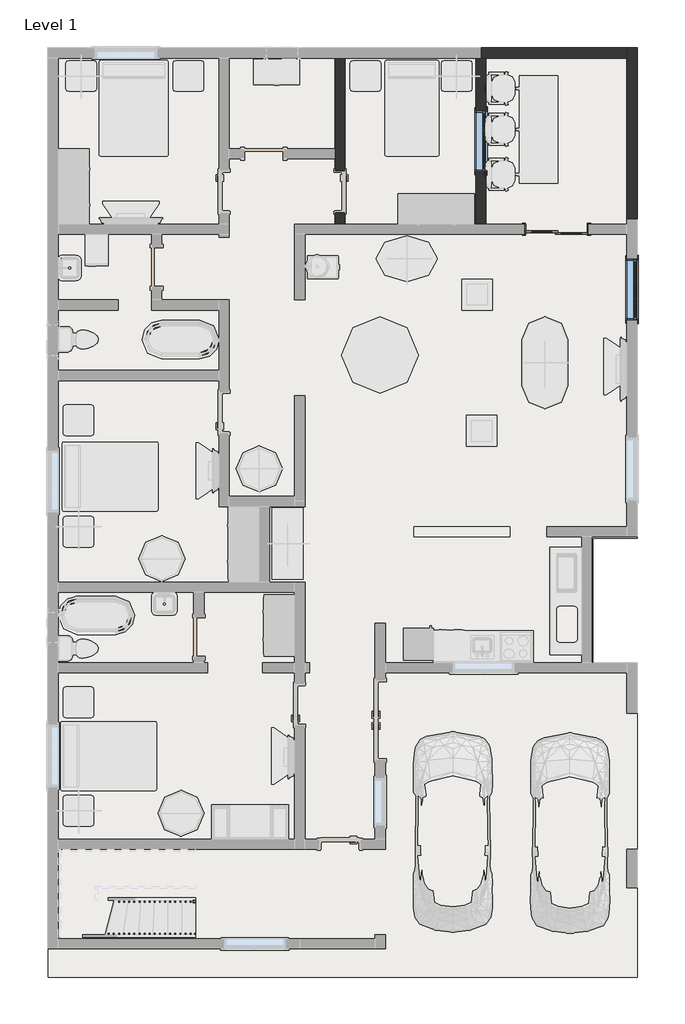
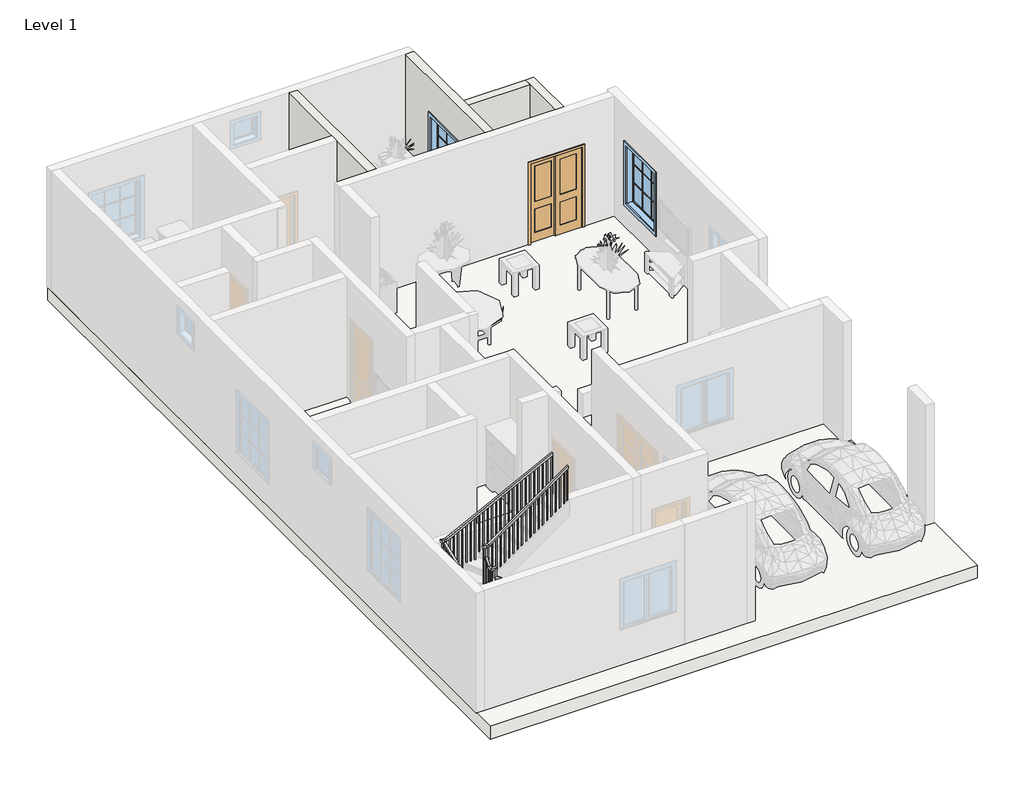
# One storey, part 2 of 3: 4 walls, 2 railings, 2 windows, 1 door, 1 slab.
"""IFC4 building model written with IfcOpenShell, lengths in millimetres."""

from ifc_helpers import new_model, si_unit, frame, origin, place, context, project, spatial, polyline, outline, extrude, faceted_brep, transform, mapped, element, save
from components import door_f9cb40a9, window_cfa1ffdd

model = new_model("IFC4")

# Units and contexts
model_context = context("Model", 3, world=origin())
ifc_project = project(units=[si_unit("LENGTHUNIT", "METRE", prefix="MILLI")], contexts=[model_context])

# Site, building, storey
site = spatial("IfcSite", under=ifc_project)
building = spatial("IfcBuilding", under=site)
storey = spatial("IfcBuildingStorey", under=building, Name="Level 1", Elevation=0.0)

# Door
placement = place(None, origin())
door_shape = door_f9cb40a9(model_context)
element("IfcDoor", 1, ObjectType="Door-Interior-Double-Sliding-2_Panel-Wood : 48\" x 80\"", at=placement, inside=storey, context=model_context, shape_type="MappedRepresentation", body=[
    mapped(door_shape, transform((-3472.131213, 10396.0883056, 0.0), x_axis=(-1.0, 0.0, 0.0), y_axis=(0.0, -1.0, 0.0), z_axis=(0.0, 0.0, 1.0))),
])

# Railings
element("IfcRailing", 2, ObjectType="Handrail - Rectangular", at=placement, inside=storey, context=model_context, shape_type="SolidModel", body=[
    faceted_brep([(-10636.560337, -2964.1366944, 1228.5737673), (-10636.560337, -2964.1366944, 1166.746771), (-10636.560337, -2913.3366944, 1166.746771), (-10636.560337, -2913.3366944, 1228.5737673), (-12557.731213, -2964.1366944, 2561.3343732), (-12608.531213, -2964.1366944, 2534.7485102), (-12608.531213, -2913.3366944, 2534.7485102), (-12557.731213, -2913.3366944, 2561.3343732), (-12557.731213, -2964.1366944, 2783.0416442), (-12608.531213, -2964.1366944, 2732.2416442), (-12608.531213, -2913.3366944, 2732.2416442), (-12557.731213, -2913.3366944, 2783.0416442), (-12684.731213, -2964.1366944, 2783.0416442), (-12684.731213, -2964.1366944, 2732.2416442), (-12633.931213, -2913.3366944, 2732.2416442), (-12633.931213, -2913.3366944, 2783.0416442), (-12684.731213, -2837.1366944, 2783.0416442), (-12684.731213, -2812.8013323, 2732.2416442), (-12633.931213, -2812.8013323, 2732.2416442), (-12633.931213, -2837.1366944, 2783.0416442), (-12684.731213, -2710.1366944, 2940.9571956), (-12684.731213, -2659.3366944, 2923.0641081), (-12633.931213, -2659.3366944, 2923.0641081), (-12633.931213, -2710.1366944, 2940.9571956), (-12684.731213, -2710.1366944, 3165.2815063), (-12684.731213, -2659.3366944, 3114.4815063), (-12633.931213, -2659.3366944, 3114.4815063), (-12633.931213, -2710.1366944, 3165.2815063), (-12684.731213, -2583.1366944, 3165.2815063), (-12684.731213, -2583.1366944, 3114.4815063), (-12633.931213, -2633.9366944, 3114.4815063), (-12633.931213, -2633.9366944, 3165.2815063), (-12557.731213, -2583.1366944, 3165.2815063), (-12541.785836, -2583.1366944, 3114.4815063), (-12541.785836, -2633.9366944, 3114.4815063), (-12557.731213, -2633.9366944, 3165.2815063), (-10647.3488243, -2583.1366944, 4495.6355204), (-10647.3488243, -2633.9366944, 4495.6355204), (-10647.3488243, -2633.9366944, 4433.7314627), (-10647.3488243, -2583.1366944, 4433.7314627)], [[[0, 1, 2, 3]], [[1, 0, 4, 5]], [[2, 1, 5, 6]], [[3, 2, 6, 7]], [[0, 3, 7, 4]], [[5, 4, 8, 9]], [[6, 5, 9, 10]], [[7, 6, 10, 11]], [[4, 7, 11, 8]], [[9, 8, 12, 13]], [[10, 9, 13, 14]], [[11, 10, 14, 15]], [[8, 11, 15, 12]], [[13, 12, 16, 17]], [[14, 13, 17, 18]], [[15, 14, 18, 19]], [[12, 15, 19, 16]], [[17, 16, 20, 21]], [[18, 17, 21, 22]], [[19, 18, 22, 23]], [[16, 19, 23, 20]], [[21, 20, 24, 25]], [[22, 21, 25, 26]], [[23, 22, 26, 27]], [[20, 23, 27, 24]], [[25, 24, 28, 29]], [[26, 25, 29, 30]], [[27, 26, 30, 31]], [[24, 27, 31, 28]], [[29, 28, 32, 33]], [[30, 29, 33, 34]], [[31, 30, 34, 35]], [[28, 31, 35, 32]], [[36, 37, 38, 39]], [[33, 32, 36, 39]], [[34, 33, 39, 38]], [[35, 34, 38, 37]], [[32, 35, 37, 36]]]),
    extrude(outline(polyline([(4383.5520658, -10719.406213), (4370.2860075, -10738.456213), (3386.6666667, -10738.456213), (3386.6666667, -10719.406213), (4383.5520658, -10719.406213)])), frame((0.0, -2618.0616944, 0.0), z_axis=(0.0, 1.0, 0.0), x_axis=(0.0, 0.0, 1.0)), (0.0, 0.0, 1.0), 19.05),
    extrude(outline(polyline([(4312.7997553, -10821.006213), (4299.5336971, -10840.056213), (3386.6666667, -10840.056213), (3386.6666667, -10821.006213), (4312.7997553, -10821.006213)])), frame((0.0, -2618.0616944, 0.0), z_axis=(0.0, 1.0, 0.0), x_axis=(0.0, 0.0, 1.0)), (0.0, 0.0, 1.0), 19.05),
    extrude(outline(polyline([(4242.0474449, -10922.606213), (4228.7813867, -10941.656213), (3217.3333333, -10941.656213), (3217.3333333, -10922.606213), (4242.0474449, -10922.606213)])), frame((0.0, -2618.0616944, 0.0), z_axis=(0.0, 1.0, 0.0), x_axis=(0.0, 0.0, 1.0)), (0.0, 0.0, 1.0), 19.05),
    extrude(outline(polyline([(4171.2951344, -11024.206213), (4158.0290762, -11043.256213), (3217.3333333, -11043.256213), (3217.3333333, -11024.206213), (4171.2951344, -11024.206213)])), frame((0.0, -2618.0616944, 0.0), z_axis=(0.0, 1.0, 0.0), x_axis=(0.0, 0.0, 1.0)), (0.0, 0.0, 1.0), 19.05),
    extrude(outline(polyline([(4100.542824, -11125.806213), (4087.2767658, -11144.856213), (3217.3333333, -11144.856213), (3217.3333333, -11125.806213), (4100.542824, -11125.806213)])), frame((0.0, -2618.0616944, 0.0), z_axis=(0.0, 1.0, 0.0), x_axis=(0.0, 0.0, 1.0)), (0.0, 0.0, 1.0), 19.05),
    extrude(outline(polyline([(4029.7905135, -11227.406213), (4016.5244553, -11246.456213), (3048.0, -11246.456213), (3048.0, -11227.406213), (4029.7905135, -11227.406213)])), frame((0.0, -2618.0616944, 0.0), z_axis=(0.0, 1.0, 0.0), x_axis=(0.0, 0.0, 1.0)), (0.0, 0.0, 1.0), 19.05),
    extrude(outline(polyline([(3959.0382031, -11329.006213), (3945.7721449, -11348.056213), (3048.0, -11348.056213), (3048.0, -11329.006213), (3959.0382031, -11329.006213)])), frame((0.0, -2618.0616944, 0.0), z_axis=(0.0, 1.0, 0.0), x_axis=(0.0, 0.0, 1.0)), (0.0, 0.0, 1.0), 19.05),
    extrude(outline(polyline([(3888.2858926, -11430.606213), (3875.0198344, -11449.656213), (3048.0, -11449.656213), (3048.0, -11430.606213), (3888.2858926, -11430.606213)])), frame((0.0, -2618.0616944, 0.0), z_axis=(0.0, 1.0, 0.0), x_axis=(0.0, 0.0, 1.0)), (0.0, 0.0, 1.0), 19.05),
    extrude(outline(polyline([(3817.5335822, -11532.206213), (3804.267524, -11551.256213), (2878.6666667, -11551.256213), (2878.6666667, -11532.206213), (3817.5335822, -11532.206213)])), frame((0.0, -2618.0616944, 0.0), z_axis=(0.0, 1.0, 0.0), x_axis=(0.0, 0.0, 1.0)), (0.0, 0.0, 1.0), 19.05),
    extrude(outline(polyline([(3746.7812717, -11633.806213), (3733.5152135, -11652.856213), (2878.6666667, -11652.856213), (2878.6666667, -11633.806213), (3746.7812717, -11633.806213)])), frame((0.0, -2618.0616944, 0.0), z_axis=(0.0, 1.0, 0.0), x_axis=(0.0, 0.0, 1.0)), (0.0, 0.0, 1.0), 19.05),
    extrude(outline(polyline([(3676.0289613, -11735.406213), (3662.7629031, -11754.456213), (2709.3333333, -11754.456213), (2709.3333333, -11735.406213), (3676.0289613, -11735.406213)])), frame((0.0, -2618.0616944, 0.0), z_axis=(0.0, 1.0, 0.0), x_axis=(0.0, 0.0, 1.0)), (0.0, 0.0, 1.0), 19.05),
    extrude(outline(polyline([(3605.2766508, -11837.006213), (3592.0105926, -11856.056213), (2709.3333333, -11856.056213), (2709.3333333, -11837.006213), (3605.2766508, -11837.006213)])), frame((0.0, -2618.0616944, 0.0), z_axis=(0.0, 1.0, 0.0), x_axis=(0.0, 0.0, 1.0)), (0.0, 0.0, 1.0), 19.05),
    extrude(outline(polyline([(3534.5243404, -11938.606213), (3521.2582822, -11957.656213), (2709.3333333, -11957.656213), (2709.3333333, -11938.606213), (3534.5243404, -11938.606213)])), frame((0.0, -2618.0616944, 0.0), z_axis=(0.0, 1.0, 0.0), x_axis=(0.0, 0.0, 1.0)), (0.0, 0.0, 1.0), 19.05),
    extrude(outline(polyline([(3463.7720299, -12040.206213), (3450.5059717, -12059.256213), (2540.0, -12059.256213), (2540.0, -12040.206213), (3463.7720299, -12040.206213)])), frame((0.0, -2618.0616944, 0.0), z_axis=(0.0, 1.0, 0.0), x_axis=(0.0, 0.0, 1.0)), (0.0, 0.0, 1.0), 19.05),
    extrude(outline(polyline([(3393.0197195, -12141.806213), (3379.7536613, -12160.856213), (2540.0, -12160.856213), (2540.0, -12141.806213), (3393.0197195, -12141.806213)])), frame((0.0, -2618.0616944, 0.0), z_axis=(0.0, 1.0, 0.0), x_axis=(0.0, 0.0, 1.0)), (0.0, 0.0, 1.0), 19.05),
    extrude(outline(polyline([(3322.267409, -12243.406213), (3309.0013508, -12262.456213), (2370.6666667, -12262.456213), (2370.6666667, -12243.406213), (3322.267409, -12243.406213)])), frame((0.0, -2618.0616944, 0.0), z_axis=(0.0, 1.0, 0.0), x_axis=(0.0, 0.0, 1.0)), (0.0, 0.0, 1.0), 19.05),
    extrude(outline(polyline([(3251.5150986, -12345.006213), (3238.2490404, -12364.056213), (2370.6666667, -12364.056213), (2370.6666667, -12345.006213), (3251.5150986, -12345.006213)])), frame((0.0, -2618.0616944, 0.0), z_axis=(0.0, 1.0, 0.0), x_axis=(0.0, 0.0, 1.0)), (0.0, 0.0, 1.0), 19.05),
    extrude(outline(polyline([(3180.7627881, -12446.606213), (3167.4967299, -12465.656213), (2201.3333333, -12465.656213), (2201.3333333, -12446.606213), (3180.7627881, -12446.606213)])), frame((0.0, -2618.0616944, 0.0), z_axis=(0.0, 1.0, 0.0), x_axis=(0.0, 0.0, 1.0)), (0.0, 0.0, 1.0), 19.05),
    extrude(outline(polyline([(-12567.256213, -2618.0616944), (-12567.256213, -2599.0116944), (-12548.206213, -2599.0116944), (-12548.206213, -2618.0616944), (-12567.256213, -2618.0616944)])), frame((0.0, 0.0, 2201.3333333), z_axis=(0.0, 0.0, 1.0), x_axis=(1.0, 0.0, 0.0)), (0.0, 0.0, 1.0), 913.1481729),
    extrude(outline(polyline([(-12649.806213, -2643.4616944), (-12668.856213, -2643.4616944), (-12668.856213, -2624.4116944), (-12649.806213, -2624.4116944), (-12649.806213, -2643.4616944)])), frame((0.0, 0.0, 2032.0), z_axis=(0.0, 0.0, 1.0), x_axis=(1.0, 0.0, 0.0)), (0.0, 0.0, 1.0), 1082.4815063),
    extrude(outline(polyline([(-2745.0616944, 2816.4711109), (-2726.0116944, 2840.1584436), (-2726.0116944, 1862.6666667), (-2745.0616944, 1862.6666667), (-2745.0616944, 2816.4711109)])), frame((-12668.856213, 0.0, 0.0), z_axis=(1.0, 0.0, 0.0), x_axis=(0.0, 1.0, 0.0)), (0.0, 0.0, 1.0), 19.05),
    extrude(outline(polyline([(-12649.806213, -2846.6616944), (-12668.856213, -2846.6616944), (-12668.856213, -2827.6116944), (-12649.806213, -2827.6116944), (-12649.806213, -2846.6616944)])), frame((0.0, 0.0, 1862.6666667), z_axis=(0.0, 0.0, 1.0), x_axis=(1.0, 0.0, 0.0)), (0.0, 0.0, 1.0), 869.5749776),
    extrude(outline(polyline([(2499.302121, -12557.435337), (2512.5175459, -12576.485337), (1524.0, -12576.485337), (1524.0, -12557.435337), (2499.302121, -12557.435337)])), frame((0.0, -2948.2616944, 0.0), z_axis=(0.0, 1.0, 0.0), x_axis=(0.0, 0.0, 1.0)), (0.0, 0.0, 1.0), 19.05),
    extrude(outline(polyline([(2428.8198545, -12455.835337), (2442.0352795, -12474.885337), (1524.0, -12474.885337), (1524.0, -12455.835337), (2428.8198545, -12455.835337)])), frame((0.0, -2948.2616944, 0.0), z_axis=(0.0, 1.0, 0.0), x_axis=(0.0, 0.0, 1.0)), (0.0, 0.0, 1.0), 19.05),
    extrude(outline(polyline([(2358.3375881, -12354.235337), (2371.553013, -12373.285337), (1354.6666667, -12373.285337), (1354.6666667, -12354.235337), (2358.3375881, -12354.235337)])), frame((0.0, -2948.2616944, 0.0), z_axis=(0.0, 1.0, 0.0), x_axis=(0.0, 0.0, 1.0)), (0.0, 0.0, 1.0), 19.05),
    extrude(outline(polyline([(2287.8553216, -12252.635337), (2301.0707466, -12271.685337), (1354.6666667, -12271.685337), (1354.6666667, -12252.635337), (2287.8553216, -12252.635337)])), frame((0.0, -2948.2616944, 0.0), z_axis=(0.0, 1.0, 0.0), x_axis=(0.0, 0.0, 1.0)), (0.0, 0.0, 1.0), 19.05),
    extrude(outline(polyline([(2217.3730552, -12151.035337), (2230.5884801, -12170.085337), (1185.3333333, -12170.085337), (1185.3333333, -12151.035337), (2217.3730552, -12151.035337)])), frame((0.0, -2948.2616944, 0.0), z_axis=(0.0, 1.0, 0.0), x_axis=(0.0, 0.0, 1.0)), (0.0, 0.0, 1.0), 19.05),
    extrude(outline(polyline([(2146.8907887, -12049.435337), (2160.1062137, -12068.485337), (1185.3333333, -12068.485337), (1185.3333333, -12049.435337), (2146.8907887, -12049.435337)])), frame((0.0, -2948.2616944, 0.0), z_axis=(0.0, 1.0, 0.0), x_axis=(0.0, 0.0, 1.0)), (0.0, 0.0, 1.0), 19.05),
    extrude(outline(polyline([(2076.4085223, -11947.835337), (2089.6239473, -11966.885337), (1016.0, -11966.885337), (1016.0, -11947.835337), (2076.4085223, -11947.835337)])), frame((0.0, -2948.2616944, 0.0), z_axis=(0.0, 1.0, 0.0), x_axis=(0.0, 0.0, 1.0)), (0.0, 0.0, 1.0), 19.05),
    extrude(outline(polyline([(2005.9262558, -11846.235337), (2019.1416808, -11865.285337), (1016.0, -11865.285337), (1016.0, -11846.235337), (2005.9262558, -11846.235337)])), frame((0.0, -2948.2616944, 0.0), z_axis=(0.0, 1.0, 0.0), x_axis=(0.0, 0.0, 1.0)), (0.0, 0.0, 1.0), 19.05),
    extrude(outline(polyline([(1935.4439894, -11744.635337), (1948.6594144, -11763.685337), (1016.0, -11763.685337), (1016.0, -11744.635337), (1935.4439894, -11744.635337)])), frame((0.0, -2948.2616944, 0.0), z_axis=(0.0, 1.0, 0.0), x_axis=(0.0, 0.0, 1.0)), (0.0, 0.0, 1.0), 19.05),
    extrude(outline(polyline([(1864.961723, -11643.035337), (1878.1771479, -11662.085337), (846.6666667, -11662.085337), (846.6666667, -11643.035337), (1864.961723, -11643.035337)])), frame((0.0, -2948.2616944, 0.0), z_axis=(0.0, 1.0, 0.0), x_axis=(0.0, 0.0, 1.0)), (0.0, 0.0, 1.0), 19.05),
    extrude(outline(polyline([(1794.4794565, -11541.435337), (1807.6948815, -11560.485337), (846.6666667, -11560.485337), (846.6666667, -11541.435337), (1794.4794565, -11541.435337)])), frame((0.0, -2948.2616944, 0.0), z_axis=(0.0, 1.0, 0.0), x_axis=(0.0, 0.0, 1.0)), (0.0, 0.0, 1.0), 19.05),
    extrude(outline(polyline([(1723.9971901, -11439.835337), (1737.212615, -11458.885337), (677.3333333, -11458.885337), (677.3333333, -11439.835337), (1723.9971901, -11439.835337)])), frame((0.0, -2948.2616944, 0.0), z_axis=(0.0, 1.0, 0.0), x_axis=(0.0, 0.0, 1.0)), (0.0, 0.0, 1.0), 19.05),
    extrude(outline(polyline([(1653.4594671, -11338.235337), (1666.674892, -11357.285337), (677.3333333, -11357.285337), (677.3333333, -11338.235337), (1653.4594671, -11338.235337)])), frame((0.0, -2948.2616944, 0.0), z_axis=(0.0, 1.0, 0.0), x_axis=(0.0, 0.0, 1.0)), (0.0, 0.0, 1.0), 19.05),
    extrude(outline(polyline([(1583.0326572, -11236.635337), (1596.2480821, -11255.685337), (677.3333333, -11255.685337), (677.3333333, -11236.635337), (1583.0326572, -11236.635337)])), frame((0.0, -2948.2616944, 0.0), z_axis=(0.0, 1.0, 0.0), x_axis=(0.0, 0.0, 1.0)), (0.0, 0.0, 1.0), 19.05),
    extrude(outline(polyline([(1512.5503907, -11135.035337), (1525.7658157, -11154.085337), (508.0, -11154.085337), (508.0, -11135.035337), (1512.5503907, -11135.035337)])), frame((0.0, -2948.2616944, 0.0), z_axis=(0.0, 1.0, 0.0), x_axis=(0.0, 0.0, 1.0)), (0.0, 0.0, 1.0), 19.05),
    extrude(outline(polyline([(1442.0681243, -11033.435337), (1455.2835492, -11052.485337), (508.0, -11052.485337), (508.0, -11033.435337), (1442.0681243, -11033.435337)])), frame((0.0, -2948.2616944, 0.0), z_axis=(0.0, 1.0, 0.0), x_axis=(0.0, 0.0, 1.0)), (0.0, 0.0, 1.0), 19.05),
    extrude(outline(polyline([(1371.5858578, -10931.835337), (1384.8012828, -10950.885337), (508.0, -10950.885337), (508.0, -10931.835337), (1371.5858578, -10931.835337)])), frame((0.0, -2948.2616944, 0.0), z_axis=(0.0, 1.0, 0.0), x_axis=(0.0, 0.0, 1.0)), (0.0, 0.0, 1.0), 19.05),
    extrude(outline(polyline([(1301.1035914, -10830.235337), (1314.3190164, -10849.285337), (338.6666667, -10849.285337), (338.6666667, -10830.235337), (1301.1035914, -10830.235337)])), frame((0.0, -2948.2616944, 0.0), z_axis=(0.0, 1.0, 0.0), x_axis=(0.0, 0.0, 1.0)), (0.0, 0.0, 1.0), 19.05),
    extrude(outline(polyline([(1230.6213249, -10728.635337), (1243.8367499, -10747.685337), (338.6666667, -10747.685337), (338.6666667, -10728.635337), (1230.6213249, -10728.635337)])), frame((0.0, -2948.2616944, 0.0), z_axis=(0.0, 1.0, 0.0), x_axis=(0.0, 0.0, 1.0)), (0.0, 0.0, 1.0), 19.05),
    extrude(outline(polyline([(-12668.856213, -2618.0616944), (-12668.856213, -2599.0116944), (-12649.806213, -2599.0116944), (-12649.806213, -2618.0616944), (-12668.856213, -2618.0616944)])), frame((0.0, 0.0, 2032.0), z_axis=(0.0, 0.0, 1.0), x_axis=(1.0, 0.0, 0.0)), (0.0, 0.0, 1.0), 1082.4815063),
    extrude(outline(polyline([(-12649.806213, -2948.2616944), (-12668.856213, -2948.2616944), (-12668.856213, -2929.2116944), (-12649.806213, -2929.2116944), (-12649.806213, -2948.2616944)])), frame((0.0, 0.0, 1693.3333333), z_axis=(0.0, 0.0, 1.0), x_axis=(1.0, 0.0, 0.0)), (0.0, 0.0, 1.0), 1038.9083109),
    extrude(outline(polyline([(4433.7314627, -10647.3488243), (4420.4654045, -10666.3988243), (3386.6666667, -10666.3988243), (3386.6666667, -10647.3488243), (4433.7314627, -10647.3488243)])), frame((0.0, -2618.0616944, 0.0), z_axis=(0.0, 1.0, 0.0), x_axis=(0.0, 0.0, 1.0)), (0.0, 0.0, 1.0), 19.05),
    extrude(outline(polyline([(1166.746771, -10636.560337), (1179.9621959, -10655.610337), (338.6666667, -10655.610337), (338.6666667, -10636.560337), (1166.746771, -10636.560337)])), frame((0.0, -2948.2616944, 0.0), z_axis=(0.0, 1.0, 0.0), x_axis=(0.0, 0.0, 1.0)), (0.0, 0.0, 1.0), 19.05),
])
element("IfcRailing", 3, ObjectType="Handrail - Rectangular", at=placement, inside=storey, context=model_context, shape_type="SolidModel", body=[
    faceted_brep([(-10636.560337, -3599.1366944, 1280.209816), (-10636.560337, -3599.1366944, 1223.2097701), (-10636.560337, -3548.3366944, 1223.2097701), (-10636.560337, -3548.3366944, 1280.209816), (-13208.6314205, -3599.1366944, 2589.1692312), (-13220.8143489, -3599.1366944, 2538.3692312), (-13220.8143489, -3548.3366944, 2538.3692312), (-13208.6314205, -3548.3366944, 2589.1692312), (-13319.731213, -3599.1366944, 2589.1692312), (-13319.731213, -3599.1366944, 2538.3692312), (-13268.931213, -3548.3366944, 2538.3692312), (-13268.931213, -3548.3366944, 2589.1692312), (-13319.731213, -3464.8815529, 2589.1692312), (-13319.731213, -3455.0834225, 2538.3692312), (-13268.931213, -3455.0834225, 2538.3692312), (-13268.931213, -3464.8815529, 2589.1692312), (-13319.731213, -2071.8173186, 3147.3118435), (-13319.731213, -2062.0191882, 3096.5118435), (-13268.931213, -2062.0191882, 3096.5118435), (-13268.931213, -2071.8173186, 3147.3118435), (-13319.731213, -1948.1366944, 3147.3118435), (-13319.731213, -1948.1366944, 3096.5118435), (-13268.931213, -1998.9366944, 3096.5118435), (-13268.931213, -1998.9366944, 3147.3118435), (-13216.1938701, -1948.1366944, 3147.3118435), (-13204.1170851, -1948.1366944, 3096.5118435), (-13204.1170851, -1998.9366944, 3096.5118435), (-13216.1938701, -1998.9366944, 3147.3118435), (-10647.3488243, -1948.1366944, 4441.8689533), (-10647.3488243, -1998.9366944, 4441.8689533), (-10647.3488243, -1998.9366944, 4384.9829156), (-10647.3488243, -1948.1366944, 4384.9829156)], [[[0, 1, 2, 3]], [[1, 0, 4, 5]], [[2, 1, 5, 6]], [[3, 2, 6, 7]], [[0, 3, 7, 4]], [[5, 4, 8, 9]], [[6, 5, 9, 10]], [[7, 6, 10, 11]], [[4, 7, 11, 8]], [[9, 8, 12, 13]], [[10, 9, 13, 14]], [[11, 10, 14, 15]], [[8, 11, 15, 12]], [[13, 12, 16, 17]], [[14, 13, 17, 18]], [[15, 14, 18, 19]], [[12, 15, 19, 16]], [[17, 16, 20, 21]], [[18, 17, 21, 22]], [[19, 18, 22, 23]], [[16, 19, 23, 20]], [[21, 20, 24, 25]], [[22, 21, 25, 26]], [[23, 22, 26, 27]], [[20, 23, 27, 24]], [[28, 29, 30, 31]], [[25, 24, 28, 31]], [[26, 25, 31, 30]], [[27, 26, 30, 29]], [[24, 27, 29, 28]]]),
    extrude(outline(polyline([(4365.6465155, -10685.7188701), (3386.6666667, -10685.7188701), (3386.6666667, -10666.6688701), (4375.2466714, -10666.6688701), (4365.6465155, -10685.7188701)])), frame((0.0, -1983.0616944, 0.0), z_axis=(0.0, 1.0, 0.0), x_axis=(0.0, 0.0, 1.0)), (0.0, 0.0, 1.0), 19.05),
    extrude(outline(polyline([(4314.445684, -10787.3188701), (3386.6666667, -10787.3188701), (3386.6666667, -10768.2688701), (4324.0458399, -10768.2688701), (4314.445684, -10787.3188701)])), frame((0.0, -1983.0616944, 0.0), z_axis=(0.0, 1.0, 0.0), x_axis=(0.0, 0.0, 1.0)), (0.0, 0.0, 1.0), 19.05),
    extrude(outline(polyline([(4263.2448525, -10888.9188701), (3386.6666667, -10888.9188701), (3386.6666667, -10869.8688701), (4272.8450084, -10869.8688701), (4263.2448525, -10888.9188701)])), frame((0.0, -1983.0616944, 0.0), z_axis=(0.0, 1.0, 0.0), x_axis=(0.0, 0.0, 1.0)), (0.0, 0.0, 1.0), 19.05),
    extrude(outline(polyline([(4212.044021, -10990.5188701), (3217.3333333, -10990.5188701), (3217.3333333, -10971.4688701), (4221.6441769, -10971.4688701), (4212.044021, -10990.5188701)])), frame((0.0, -1983.0616944, 0.0), z_axis=(0.0, 1.0, 0.0), x_axis=(0.0, 0.0, 1.0)), (0.0, 0.0, 1.0), 19.05),
    extrude(outline(polyline([(4160.8431895, -11092.1188701), (3217.3333333, -11092.1188701), (3217.3333333, -11073.0688701), (4170.4433454, -11073.0688701), (4160.8431895, -11092.1188701)])), frame((0.0, -1983.0616944, 0.0), z_axis=(0.0, 1.0, 0.0), x_axis=(0.0, 0.0, 1.0)), (0.0, 0.0, 1.0), 19.05),
    extrude(outline(polyline([(4109.642358, -11193.7188701), (3217.3333333, -11193.7188701), (3217.3333333, -11174.6688701), (4119.2425139, -11174.6688701), (4109.642358, -11193.7188701)])), frame((0.0, -1983.0616944, 0.0), z_axis=(0.0, 1.0, 0.0), x_axis=(0.0, 0.0, 1.0)), (0.0, 0.0, 1.0), 19.05),
    extrude(outline(polyline([(4058.4415265, -11295.3188701), (3048.0, -11295.3188701), (3048.0, -11276.2688701), (4068.0416824, -11276.2688701), (4058.4415265, -11295.3188701)])), frame((0.0, -1983.0616944, 0.0), z_axis=(0.0, 1.0, 0.0), x_axis=(0.0, 0.0, 1.0)), (0.0, 0.0, 1.0), 19.05),
    extrude(outline(polyline([(4007.240695, -11396.9188701), (3048.0, -11396.9188701), (3048.0, -11377.8688701), (4016.8408509, -11377.8688701), (4007.240695, -11396.9188701)])), frame((0.0, -1983.0616944, 0.0), z_axis=(0.0, 1.0, 0.0), x_axis=(0.0, 0.0, 1.0)), (0.0, 0.0, 1.0), 19.05),
    extrude(outline(polyline([(3956.0398635, -11498.5188701), (3048.0, -11498.5188701), (3048.0, -11479.4688701), (3965.6400194, -11479.4688701), (3956.0398635, -11498.5188701)])), frame((0.0, -1983.0616944, 0.0), z_axis=(0.0, 1.0, 0.0), x_axis=(0.0, 0.0, 1.0)), (0.0, 0.0, 1.0), 19.05),
    extrude(outline(polyline([(3904.8390319, -11600.1188701), (2878.6666667, -11600.1188701), (2878.6666667, -11581.0688701), (3914.4391879, -11581.0688701), (3904.8390319, -11600.1188701)])), frame((0.0, -1983.0616944, 0.0), z_axis=(0.0, 1.0, 0.0), x_axis=(0.0, 0.0, 1.0)), (0.0, 0.0, 1.0), 19.05),
    extrude(outline(polyline([(3853.6382004, -11701.7188701), (2878.6666667, -11701.7188701), (2878.6666667, -11682.6688701), (3863.2383563, -11682.6688701), (3853.6382004, -11701.7188701)])), frame((0.0, -1983.0616944, 0.0), z_axis=(0.0, 1.0, 0.0), x_axis=(0.0, 0.0, 1.0)), (0.0, 0.0, 1.0), 19.05),
    extrude(outline(polyline([(3802.4373689, -11803.3188701), (2709.3333333, -11803.3188701), (2709.3333333, -11784.2688701), (3812.0375248, -11784.2688701), (3802.4373689, -11803.3188701)])), frame((0.0, -1983.0616944, 0.0), z_axis=(0.0, 1.0, 0.0), x_axis=(0.0, 0.0, 1.0)), (0.0, 0.0, 1.0), 19.05),
    extrude(outline(polyline([(3751.2365374, -11904.9188701), (2709.3333333, -11904.9188701), (2709.3333333, -11885.8688701), (3760.8366933, -11885.8688701), (3751.2365374, -11904.9188701)])), frame((0.0, -1983.0616944, 0.0), z_axis=(0.0, 1.0, 0.0), x_axis=(0.0, 0.0, 1.0)), (0.0, 0.0, 1.0), 19.05),
    extrude(outline(polyline([(3700.0357059, -12006.5188701), (2709.3333333, -12006.5188701), (2709.3333333, -11987.4688701), (3709.6358618, -11987.4688701), (3700.0357059, -12006.5188701)])), frame((0.0, -1983.0616944, 0.0), z_axis=(0.0, 1.0, 0.0), x_axis=(0.0, 0.0, 1.0)), (0.0, 0.0, 1.0), 19.05),
    extrude(outline(polyline([(3648.8348744, -12108.1188701), (2540.0, -12108.1188701), (2540.0, -12089.0688701), (3658.4350303, -12089.0688701), (3648.8348744, -12108.1188701)])), frame((0.0, -1983.0616944, 0.0), z_axis=(0.0, 1.0, 0.0), x_axis=(0.0, 0.0, 1.0)), (0.0, 0.0, 1.0), 19.05),
    extrude(outline(polyline([(3597.6340429, -12209.7188701), (2540.0, -12209.7188701), (2540.0, -12190.6688701), (3607.2341988, -12190.6688701), (3597.6340429, -12209.7188701)])), frame((0.0, -1983.0616944, 0.0), z_axis=(0.0, 1.0, 0.0), x_axis=(0.0, 0.0, 1.0)), (0.0, 0.0, 1.0), 19.05),
    extrude(outline(polyline([(3546.4332114, -12311.3188701), (2540.0, -12311.3188701), (2540.0, -12292.2688701), (3556.0333673, -12292.2688701), (3546.4332114, -12311.3188701)])), frame((0.0, -1983.0616944, 0.0), z_axis=(0.0, 1.0, 0.0), x_axis=(0.0, 0.0, 1.0)), (0.0, 0.0, 1.0), 19.05),
    extrude(outline(polyline([(3495.2323799, -12412.9188701), (2540.0, -12412.9188701), (2540.0, -12393.8688701), (3504.8325358, -12393.8688701), (3495.2323799, -12412.9188701)])), frame((0.0, -1983.0616944, 0.0), z_axis=(0.0, 1.0, 0.0), x_axis=(0.0, 0.0, 1.0)), (0.0, 0.0, 1.0), 19.05),
    extrude(outline(polyline([(3444.0315484, -12514.5188701), (2370.6666667, -12514.5188701), (2370.6666667, -12495.4688701), (3453.6317043, -12495.4688701), (3444.0315484, -12514.5188701)])), frame((0.0, -1983.0616944, 0.0), z_axis=(0.0, 1.0, 0.0), x_axis=(0.0, 0.0, 1.0)), (0.0, 0.0, 1.0), 19.05),
    extrude(outline(polyline([(3392.8307169, -12616.1188701), (2370.6666667, -12616.1188701), (2370.6666667, -12597.0688701), (3402.4308728, -12597.0688701), (3392.8307169, -12616.1188701)])), frame((0.0, -1983.0616944, 0.0), z_axis=(0.0, 1.0, 0.0), x_axis=(0.0, 0.0, 1.0)), (0.0, 0.0, 1.0), 19.05),
    extrude(outline(polyline([(3341.6298854, -12717.7188701), (2370.6666667, -12717.7188701), (2370.6666667, -12698.6688701), (3351.2300413, -12698.6688701), (3341.6298854, -12717.7188701)])), frame((0.0, -1983.0616944, 0.0), z_axis=(0.0, 1.0, 0.0), x_axis=(0.0, 0.0, 1.0)), (0.0, 0.0, 1.0), 19.05),
    extrude(outline(polyline([(3290.4290538, -12819.3188701), (2201.3333333, -12819.3188701), (2201.3333333, -12800.2688701), (3300.0292098, -12800.2688701), (3290.4290538, -12819.3188701)])), frame((0.0, -1983.0616944, 0.0), z_axis=(0.0, 1.0, 0.0), x_axis=(0.0, 0.0, 1.0)), (0.0, 0.0, 1.0), 19.05),
    extrude(outline(polyline([(3239.2282223, -12920.9188701), (2201.3333333, -12920.9188701), (2201.3333333, -12901.8688701), (3248.8283782, -12901.8688701), (3239.2282223, -12920.9188701)])), frame((0.0, -1983.0616944, 0.0), z_axis=(0.0, 1.0, 0.0), x_axis=(0.0, 0.0, 1.0)), (0.0, 0.0, 1.0), 19.05),
    extrude(outline(polyline([(3188.0273908, -13022.5188701), (2201.3333333, -13022.5188701), (2201.3333333, -13003.4688701), (3197.6275467, -13003.4688701), (3188.0273908, -13022.5188701)])), frame((0.0, -1983.0616944, 0.0), z_axis=(0.0, 1.0, 0.0), x_axis=(0.0, 0.0, 1.0)), (0.0, 0.0, 1.0), 19.05),
    extrude(outline(polyline([(3136.6282257, -13124.1188701), (2201.3333333, -13124.1188701), (2201.3333333, -13105.0688701), (3146.3230109, -13105.0688701), (3136.6282257, -13124.1188701)])), frame((0.0, -1983.0616944, 0.0), z_axis=(0.0, 1.0, 0.0), x_axis=(0.0, 0.0, 1.0)), (0.0, 0.0, 1.0), 19.05),
    extrude(outline(polyline([(-2134.5565529, 3067.4491533), (-2134.5565529, 2032.0), (-2153.6065529, 2032.0), (-2153.6065529, 3059.8166145), (-2134.5565529, 3067.4491533)])), frame((-13303.856213, 0.0, 0.0), z_axis=(1.0, 0.0, 0.0), x_axis=(0.0, 1.0, 0.0)), (0.0, 0.0, 1.0), 19.05),
    extrude(outline(polyline([(-2236.1565529, 3026.7422799), (-2236.1565529, 2032.0), (-2255.2065529, 2032.0), (-2255.2065529, 3019.1097411), (-2236.1565529, 3026.7422799)])), frame((-13303.856213, 0.0, 0.0), z_axis=(1.0, 0.0, 0.0), x_axis=(0.0, 1.0, 0.0)), (0.0, 0.0, 1.0), 19.05),
    extrude(outline(polyline([(-2337.7565529, 2986.0354065), (-2337.7565529, 2032.0), (-2356.8065529, 2032.0), (-2356.8065529, 2978.4028678), (-2337.7565529, 2986.0354065)])), frame((-13303.856213, 0.0, 0.0), z_axis=(1.0, 0.0, 0.0), x_axis=(0.0, 1.0, 0.0)), (0.0, 0.0, 1.0), 19.05),
    extrude(outline(polyline([(-2439.3565529, 2945.3285331), (-2439.3565529, 2032.0), (-2458.4065529, 2032.0), (-2458.4065529, 2937.6959944), (-2439.3565529, 2945.3285331)])), frame((-13303.856213, 0.0, 0.0), z_axis=(1.0, 0.0, 0.0), x_axis=(0.0, 1.0, 0.0)), (0.0, 0.0, 1.0), 19.05),
    extrude(outline(polyline([(-2540.9565529, 2904.6216597), (-2540.9565529, 2032.0), (-2560.0065529, 2032.0), (-2560.0065529, 2896.989121), (-2540.9565529, 2904.6216597)])), frame((-13303.856213, 0.0, 0.0), z_axis=(1.0, 0.0, 0.0), x_axis=(0.0, 1.0, 0.0)), (0.0, 0.0, 1.0), 19.05),
    extrude(outline(polyline([(-2642.5565529, 2863.9147864), (-2642.5565529, 1862.6666667), (-2661.6065529, 1862.6666667), (-2661.6065529, 2856.2822476), (-2642.5565529, 2863.9147864)])), frame((-13303.856213, 0.0, 0.0), z_axis=(1.0, 0.0, 0.0), x_axis=(0.0, 1.0, 0.0)), (0.0, 0.0, 1.0), 19.05),
    extrude(outline(polyline([(-2744.1565529, 2823.207913), (-2744.1565529, 1862.6666667), (-2763.2065529, 1862.6666667), (-2763.2065529, 2815.5753742), (-2744.1565529, 2823.207913)])), frame((-13303.856213, 0.0, 0.0), z_axis=(1.0, 0.0, 0.0), x_axis=(0.0, 1.0, 0.0)), (0.0, 0.0, 1.0), 19.05),
    extrude(outline(polyline([(-2845.7565529, 2782.5010396), (-2845.7565529, 1862.6666667), (-2864.8065529, 1862.6666667), (-2864.8065529, 2774.8685008), (-2845.7565529, 2782.5010396)])), frame((-13303.856213, 0.0, 0.0), z_axis=(1.0, 0.0, 0.0), x_axis=(0.0, 1.0, 0.0)), (0.0, 0.0, 1.0), 19.05),
    extrude(outline(polyline([(-2947.3565529, 2741.7941662), (-2947.3565529, 1862.6666667), (-2966.4065529, 1862.6666667), (-2966.4065529, 2734.1616274), (-2947.3565529, 2741.7941662)])), frame((-13303.856213, 0.0, 0.0), z_axis=(1.0, 0.0, 0.0), x_axis=(0.0, 1.0, 0.0)), (0.0, 0.0, 1.0), 19.05),
    extrude(outline(polyline([(-3048.9565529, 2701.0872928), (-3048.9565529, 1693.3333333), (-3068.0065529, 1693.3333333), (-3068.0065529, 2693.4547541), (-3048.9565529, 2701.0872928)])), frame((-13303.856213, 0.0, 0.0), z_axis=(1.0, 0.0, 0.0), x_axis=(0.0, 1.0, 0.0)), (0.0, 0.0, 1.0), 19.05),
    extrude(outline(polyline([(-3150.5565529, 2660.3804194), (-3150.5565529, 1693.3333333), (-3169.6065529, 1693.3333333), (-3169.6065529, 2652.7478807), (-3150.5565529, 2660.3804194)])), frame((-13303.856213, 0.0, 0.0), z_axis=(1.0, 0.0, 0.0), x_axis=(0.0, 1.0, 0.0)), (0.0, 0.0, 1.0), 19.05),
    extrude(outline(polyline([(-3252.1565529, 2619.673546), (-3252.1565529, 1693.3333333), (-3271.2065529, 1693.3333333), (-3271.2065529, 2612.0410073), (-3252.1565529, 2619.673546)])), frame((-13303.856213, 0.0, 0.0), z_axis=(1.0, 0.0, 0.0), x_axis=(0.0, 1.0, 0.0)), (0.0, 0.0, 1.0), 19.05),
    extrude(outline(polyline([(-3353.7565529, 2578.9666727), (-3353.7565529, 1693.3333333), (-3372.8065529, 1693.3333333), (-3372.8065529, 2571.3341339), (-3353.7565529, 2578.9666727)])), frame((-13303.856213, 0.0, 0.0), z_axis=(1.0, 0.0, 0.0), x_axis=(0.0, 1.0, 0.0)), (0.0, 0.0, 1.0), 19.05),
    extrude(outline(polyline([(-13303.856213, -3481.6616944), (-13303.856213, -3462.6116944), (-13284.806213, -3462.6116944), (-13284.806213, -3481.6616944), (-13303.856213, -3481.6616944)])), frame((0.0, 0.0, 1693.3333333), z_axis=(0.0, 0.0, 1.0), x_axis=(1.0, 0.0, 0.0)), (0.0, 0.0, 1.0), 845.0358979),
    extrude(outline(polyline([(2520.695199, -13186.085337), (1524.0, -13186.085337), (1524.0, -13167.035337), (2511.0004138, -13167.035337), (2520.695199, -13186.085337)])), frame((0.0, -3583.2616944, 0.0), z_axis=(0.0, 1.0, 0.0), x_axis=(0.0, 0.0, 1.0)), (0.0, 0.0, 1.0), 19.05),
    extrude(outline(polyline([(2468.9896776, -13084.485337), (1524.0, -13084.485337), (1524.0, -13065.435337), (2459.2948923, -13065.435337), (2468.9896776, -13084.485337)])), frame((0.0, -3583.2616944, 0.0), z_axis=(0.0, 1.0, 0.0), x_axis=(0.0, 0.0, 1.0)), (0.0, 0.0, 1.0), 19.05),
    extrude(outline(polyline([(2417.2841561, -12982.885337), (1524.0, -12982.885337), (1524.0, -12963.835337), (2407.5893709, -12963.835337), (2417.2841561, -12982.885337)])), frame((0.0, -3583.2616944, 0.0), z_axis=(0.0, 1.0, 0.0), x_axis=(0.0, 0.0, 1.0)), (0.0, 0.0, 1.0), 19.05),
    extrude(outline(polyline([(2365.5786347, -12881.285337), (1524.0, -12881.285337), (1524.0, -12862.235337), (2355.8838494, -12862.235337), (2365.5786347, -12881.285337)])), frame((0.0, -3583.2616944, 0.0), z_axis=(0.0, 1.0, 0.0), x_axis=(0.0, 0.0, 1.0)), (0.0, 0.0, 1.0), 19.05),
    extrude(outline(polyline([(2313.8731132, -12779.685337), (1524.0, -12779.685337), (1524.0, -12760.635337), (2304.178328, -12760.635337), (2313.8731132, -12779.685337)])), frame((0.0, -3583.2616944, 0.0), z_axis=(0.0, 1.0, 0.0), x_axis=(0.0, 0.0, 1.0)), (0.0, 0.0, 1.0), 19.05),
    extrude(outline(polyline([(2262.1675918, -12678.085337), (1354.6666667, -12678.085337), (1354.6666667, -12659.035337), (2252.4728065, -12659.035337), (2262.1675918, -12678.085337)])), frame((0.0, -3583.2616944, 0.0), z_axis=(0.0, 1.0, 0.0), x_axis=(0.0, 0.0, 1.0)), (0.0, 0.0, 1.0), 19.05),
    extrude(outline(polyline([(2210.4620703, -12576.485337), (1354.6666667, -12576.485337), (1354.6666667, -12557.435337), (2200.767285, -12557.435337), (2210.4620703, -12576.485337)])), frame((0.0, -3583.2616944, 0.0), z_axis=(0.0, 1.0, 0.0), x_axis=(0.0, 0.0, 1.0)), (0.0, 0.0, 1.0), 19.05),
    extrude(outline(polyline([(2158.7565489, -12474.885337), (1354.6666667, -12474.885337), (1354.6666667, -12455.835337), (2149.0617636, -12455.835337), (2158.7565489, -12474.885337)])), frame((0.0, -3583.2616944, 0.0), z_axis=(0.0, 1.0, 0.0), x_axis=(0.0, 0.0, 1.0)), (0.0, 0.0, 1.0), 19.05),
    extrude(outline(polyline([(2107.0510274, -12373.285337), (1185.3333333, -12373.285337), (1185.3333333, -12354.235337), (2097.3562421, -12354.235337), (2107.0510274, -12373.285337)])), frame((0.0, -3583.2616944, 0.0), z_axis=(0.0, 1.0, 0.0), x_axis=(0.0, 0.0, 1.0)), (0.0, 0.0, 1.0), 19.05),
    extrude(outline(polyline([(2055.345506, -12271.685337), (1185.3333333, -12271.685337), (1185.3333333, -12252.635337), (2045.6507207, -12252.635337), (2055.345506, -12271.685337)])), frame((0.0, -3583.2616944, 0.0), z_axis=(0.0, 1.0, 0.0), x_axis=(0.0, 0.0, 1.0)), (0.0, 0.0, 1.0), 19.05),
    extrude(outline(polyline([(2003.6399845, -12170.085337), (1185.3333333, -12170.085337), (1185.3333333, -12151.035337), (1993.9451992, -12151.035337), (2003.6399845, -12170.085337)])), frame((0.0, -3583.2616944, 0.0), z_axis=(0.0, 1.0, 0.0), x_axis=(0.0, 0.0, 1.0)), (0.0, 0.0, 1.0), 19.05),
    extrude(outline(polyline([(1951.9344631, -12068.485337), (1016.0, -12068.485337), (1016.0, -12049.435337), (1942.2396778, -12049.435337), (1951.9344631, -12068.485337)])), frame((0.0, -3583.2616944, 0.0), z_axis=(0.0, 1.0, 0.0), x_axis=(0.0, 0.0, 1.0)), (0.0, 0.0, 1.0), 19.05),
    extrude(outline(polyline([(1900.2289416, -11966.885337), (1016.0, -11966.885337), (1016.0, -11947.835337), (1890.5341563, -11947.835337), (1900.2289416, -11966.885337)])), frame((0.0, -3583.2616944, 0.0), z_axis=(0.0, 1.0, 0.0), x_axis=(0.0, 0.0, 1.0)), (0.0, 0.0, 1.0), 19.05),
    extrude(outline(polyline([(1848.5234201, -11865.285337), (1016.0, -11865.285337), (1016.0, -11846.235337), (1838.8286349, -11846.235337), (1848.5234201, -11865.285337)])), frame((0.0, -3583.2616944, 0.0), z_axis=(0.0, 1.0, 0.0), x_axis=(0.0, 0.0, 1.0)), (0.0, 0.0, 1.0), 19.05),
    extrude(outline(polyline([(1796.8178987, -11763.685337), (846.6666667, -11763.685337), (846.6666667, -11744.635337), (1787.1231134, -11744.635337), (1796.8178987, -11763.685337)])), frame((0.0, -3583.2616944, 0.0), z_axis=(0.0, 1.0, 0.0), x_axis=(0.0, 0.0, 1.0)), (0.0, 0.0, 1.0), 19.05),
    extrude(outline(polyline([(1745.1123772, -11662.085337), (846.6666667, -11662.085337), (846.6666667, -11643.035337), (1735.417592, -11643.035337), (1745.1123772, -11662.085337)])), frame((0.0, -3583.2616944, 0.0), z_axis=(0.0, 1.0, 0.0), x_axis=(0.0, 0.0, 1.0)), (0.0, 0.0, 1.0), 19.05),
    extrude(outline(polyline([(1693.4068558, -11560.485337), (846.6666667, -11560.485337), (846.6666667, -11541.435337), (1683.7120705, -11541.435337), (1693.4068558, -11560.485337)])), frame((0.0, -3583.2616944, 0.0), z_axis=(0.0, 1.0, 0.0), x_axis=(0.0, 0.0, 1.0)), (0.0, 0.0, 1.0), 19.05),
    extrude(outline(polyline([(1641.7013343, -11458.885337), (677.3333333, -11458.885337), (677.3333333, -11439.835337), (1632.0065491, -11439.835337), (1641.7013343, -11458.885337)])), frame((0.0, -3583.2616944, 0.0), z_axis=(0.0, 1.0, 0.0), x_axis=(0.0, 0.0, 1.0)), (0.0, 0.0, 1.0), 19.05),
    extrude(outline(polyline([(1589.9958129, -11357.285337), (677.3333333, -11357.285337), (677.3333333, -11338.235337), (1580.3010276, -11338.235337), (1589.9958129, -11357.285337)])), frame((0.0, -3583.2616944, 0.0), z_axis=(0.0, 1.0, 0.0), x_axis=(0.0, 0.0, 1.0)), (0.0, 0.0, 1.0), 19.05),
    extrude(outline(polyline([(1538.2902914, -11255.685337), (677.3333333, -11255.685337), (677.3333333, -11236.635337), (1528.5955061, -11236.635337), (1538.2902914, -11255.685337)])), frame((0.0, -3583.2616944, 0.0), z_axis=(0.0, 1.0, 0.0), x_axis=(0.0, 0.0, 1.0)), (0.0, 0.0, 1.0), 19.05),
    extrude(outline(polyline([(1486.58477, -11154.085337), (508.0, -11154.085337), (508.0, -11135.035337), (1476.8899847, -11135.035337), (1486.58477, -11154.085337)])), frame((0.0, -3583.2616944, 0.0), z_axis=(0.0, 1.0, 0.0), x_axis=(0.0, 0.0, 1.0)), (0.0, 0.0, 1.0), 19.05),
    extrude(outline(polyline([(1434.8792485, -11052.485337), (508.0, -11052.485337), (508.0, -11033.435337), (1425.1844632, -11033.435337), (1434.8792485, -11052.485337)])), frame((0.0, -3583.2616944, 0.0), z_axis=(0.0, 1.0, 0.0), x_axis=(0.0, 0.0, 1.0)), (0.0, 0.0, 1.0), 19.05),
    extrude(outline(polyline([(1383.1737271, -10950.885337), (508.0, -10950.885337), (508.0, -10931.835337), (1373.4789418, -10931.835337), (1383.1737271, -10950.885337)])), frame((0.0, -3583.2616944, 0.0), z_axis=(0.0, 1.0, 0.0), x_axis=(0.0, 0.0, 1.0)), (0.0, 0.0, 1.0), 19.05),
    extrude(outline(polyline([(1331.4682056, -10849.285337), (338.6666667, -10849.285337), (338.6666667, -10830.235337), (1321.7734203, -10830.235337), (1331.4682056, -10849.285337)])), frame((0.0, -3583.2616944, 0.0), z_axis=(0.0, 1.0, 0.0), x_axis=(0.0, 0.0, 1.0)), (0.0, 0.0, 1.0), 19.05),
    extrude(outline(polyline([(1279.7626842, -10747.685337), (338.6666667, -10747.685337), (338.6666667, -10728.635337), (1270.0678989, -10728.635337), (1279.7626842, -10747.685337)])), frame((0.0, -3583.2616944, 0.0), z_axis=(0.0, 1.0, 0.0), x_axis=(0.0, 0.0, 1.0)), (0.0, 0.0, 1.0), 19.05),
    extrude(outline(polyline([(-13225.7188701, -1964.0116944), (-13206.6688701, -1964.0116944), (-13206.6688701, -1983.0616944), (-13225.7188701, -1983.0616944), (-13225.7188701, -1964.0116944)])), frame((0.0, 0.0, 2201.3333333), z_axis=(0.0, 0.0, 1.0), x_axis=(1.0, 0.0, 0.0)), (0.0, 0.0, 1.0), 895.1785101),
    extrude(outline(polyline([(-13303.856213, -1983.0616944), (-13303.856213, -1964.0116944), (-13284.806213, -1964.0116944), (-13284.806213, -1983.0616944), (-13303.856213, -1983.0616944)])), frame((0.0, 0.0, 2032.0), z_axis=(0.0, 0.0, 1.0), x_axis=(1.0, 0.0, 0.0)), (0.0, 0.0, 1.0), 1064.5118435),
    extrude(outline(polyline([(-2062.2923186, 3096.4024115), (-2062.2923186, 2032.0), (-2081.3423186, 2032.0), (-2081.3423186, 3088.7698728), (-2062.2923186, 3096.4024115)])), frame((-13303.856213, 0.0, 0.0), z_axis=(1.0, 0.0, 0.0), x_axis=(0.0, 1.0, 0.0)), (0.0, 0.0, 1.0), 19.05),
    extrude(outline(polyline([(-13303.856213, -3474.4065529), (-13303.856213, -3455.3565529), (-13284.806213, -3455.3565529), (-13284.806213, -3474.4065529), (-13303.856213, -3474.4065529)])), frame((0.0, 0.0, 1693.3333333), z_axis=(0.0, 0.0, 1.0), x_axis=(1.0, 0.0, 0.0)), (0.0, 0.0, 1.0), 845.0358979),
    extrude(outline(polyline([(-13284.806213, -3583.2616944), (-13303.856213, -3583.2616944), (-13303.856213, -3564.2116944), (-13284.806213, -3564.2116944), (-13284.806213, -3583.2616944)])), frame((0.0, 0.0, 1693.3333333), z_axis=(0.0, 0.0, 1.0), x_axis=(1.0, 0.0, 0.0)), (0.0, 0.0, 1.0), 845.0358979),
    extrude(outline(polyline([(2537.0165779, -13218.1564205), (1524.0, -13218.1564205), (1524.0, -13199.1064205), (2527.3217926, -13199.1064205), (2537.0165779, -13218.1564205)])), frame((0.0, -3583.2616944, 0.0), z_axis=(0.0, 1.0, 0.0), x_axis=(0.0, 0.0, 1.0)), (0.0, 0.0, 1.0), 19.05),
    extrude(outline(polyline([(4375.3827597, -10666.3988243), (3386.6666667, -10666.3988243), (3386.6666667, -10647.3488243), (4384.9829156, -10647.3488243), (4375.3827597, -10666.3988243)])), frame((0.0, -1983.0616944, 0.0), z_axis=(0.0, 1.0, 0.0), x_axis=(0.0, 0.0, 1.0)), (0.0, 0.0, 1.0), 19.05),
    extrude(outline(polyline([(1232.9045553, -10655.610337), (338.6666667, -10655.610337), (338.6666667, -10636.560337), (1223.2097701, -10636.560337), (1232.9045553, -10655.610337)])), frame((0.0, -3583.2616944, 0.0), z_axis=(0.0, 1.0, 0.0), x_axis=(0.0, 0.0, 1.0)), (0.0, 0.0, 1.0), 19.05),
])

# Slab
element("IfcSlab", 4, at=placement, inside=storey, context=model_context, shape_type="SweptSolid", body=[
    extrude(outline(polyline([(-1864.181213, 13956.4133056), (-1864.181213, 4267.0133056), (-2753.181213, 4267.0133056), (-2753.181213, 1803.2133056), (-1864.181213, 1803.2133056), (-1864.181213, -4445.1866944), (-13567.381213, -4445.1866944), (-13567.381213, 13956.4133056), (-1864.181213, 13956.4133056)])), frame((0.0, 0.0, -323.85), z_axis=(0.0, 0.0, 1.0), x_axis=(1.0, 0.0, 0.0)), (0.0, 0.0, 1.0), 323.85),
])

# Walls
element("IfcWall", 5, ObjectType="Generic - 8\"", at=placement, inside=storey, context=model_context, shape_type="Brep", body=[
    faceted_brep([(-5073.731213, 13797.6633056, 3048.0), (-5073.731213, 13797.6633056, 0.0), (-5073.731213, 10500.8633056, 0.0), (-5073.731213, 10500.8633056, 3048.0), (-5073.731213, 11539.6633056, 2133.6), (-5073.731213, 11539.6633056, 609.6), (-5073.731213, 12758.8633056, 609.6), (-5073.731213, 12758.8633056, 2133.6), (-4870.531213, 13797.6633056, 0.0), (-4870.531213, 13797.6633056, 1219.2), (-4870.531213, 13797.6633056, 3048.0), (-4870.531213, 10500.8633056, 3048.0), (-4870.531213, 10500.8633056, 0.0), (-4870.531213, 11539.6633056, 2133.6), (-4870.531213, 12758.8633056, 2133.6), (-4870.531213, 12758.8633056, 609.6), (-4870.531213, 11539.6633056, 609.6), (-4972.131213, 13797.6633056, 0.0)], [[[0, 1, 2, 3], [4, 5, 6, 7]], [[8, 9, 10, 11, 12], [13, 14, 15, 16]], [[2, 1, 17, 8, 12]], [[3, 2, 12, 11]], [[0, 10, 9, 8, 17, 1]], [[5, 4, 13, 16]], [[6, 5, 16, 15]], [[7, 6, 15, 14]], [[4, 7, 14, 13]], [[0, 3, 11, 10]]]),
])
element("IfcWall", 6, ObjectType="Generic - 8\"", at=placement, inside=storey, context=model_context, shape_type="Brep", body=[
    faceted_brep([(-7670.531213, 10500.8633056, 3048.0), (-7670.531213, 10500.8633056, 0.0), (-7670.531213, 10742.8633056, 0.0), (-7670.531213, 10742.8633056, 2057.4), (-7670.531213, 11555.6633056, 2057.4), (-7670.531213, 11555.6633056, 0.0), (-7670.531213, 13797.6633056, 0.0), (-7670.531213, 13797.6633056, 3048.0), (-7873.731213, 10500.8633056, 0.0), (-7873.731213, 10500.8633056, 3048.0), (-7873.731213, 11797.6633056, 3048.0), (-7873.731213, 12000.8633056, 3048.0), (-7873.731213, 13797.6633056, 3048.0), (-7873.731213, 13797.6633056, 0.0), (-7873.731213, 12000.8633056, 0.0), (-7873.731213, 11797.6633056, 0.0), (-7873.731213, 11555.6633056, 0.0), (-7873.731213, 11555.6633056, 2057.4), (-7873.731213, 10742.8633056, 2057.4), (-7873.731213, 10742.8633056, 0.0)], [[[0, 1, 2, 3, 4, 5, 6, 7]], [[8, 9, 10, 11, 12, 13, 14, 15, 16, 17, 18, 19]], [[1, 8, 19, 2]], [[13, 6, 5, 16, 15, 14]], [[1, 0, 9, 8]], [[7, 6, 13, 12]], [[4, 17, 16, 5]], [[17, 4, 3, 18]], [[18, 3, 2, 19]], [[0, 7, 12, 11, 10, 9]]]),
])
element("IfcWall", 7, ObjectType="Generic - 8\"", at=placement, inside=storey, context=model_context, shape_type="Brep", body=[
    faceted_brep([(-2073.731213, 14000.8633056, 0.0), (-2073.731213, 13797.6633056, 0.0), (-2073.731213, 10597.2633056, 0.0), (-2073.731213, 10597.2633056, 1219.2), (-2073.731213, 13797.6633056, 1219.2), (-2073.731213, 14000.8633056, 1219.2), (-1870.531213, 14000.8633056, 0.0), (-1870.531213, 14000.8633056, 1219.2), (-1870.531213, 10597.2633056, 1219.2), (-1870.531213, 10597.2633056, 0.0)], [[[0, 1, 2, 3, 4, 5]], [[6, 7, 8, 9]], [[2, 1, 0, 6, 9]], [[3, 2, 9, 8]], [[5, 4, 3, 8, 7]], [[0, 5, 7, 6]]]),
])
element("IfcWall", 8, ObjectType="Generic - 8\"", at=placement, inside=storey, context=model_context, shape_type="Brep", body=[
    faceted_brep([(-4972.131213, 13797.6633056, 0.0), (-4870.531213, 13797.6633056, 0.0), (-2073.731213, 13797.6633056, 0.0), (-2073.731213, 13797.6633056, 1219.2), (-4870.531213, 13797.6633056, 1219.2), (-4972.131213, 13797.6633056, 1219.2), (-4972.131213, 14000.8633056, 0.0), (-4972.131213, 14000.8633056, 1219.2), (-4870.531213, 14000.8633056, 1219.2), (-2073.731213, 14000.8633056, 1219.2), (-2073.731213, 14000.8633056, 0.0)], [[[0, 1, 2, 3, 4, 5]], [[6, 7, 8, 9, 10]], [[2, 1, 0, 6, 10]], [[5, 4, 3, 9, 8, 7]], [[0, 5, 7, 6]], [[3, 2, 10, 9]]]),
])

# Windows
window_shape = window_cfa1ffdd(model_context)
element("IfcWindow", 9, ObjectType="Casement 3x3 with Trim : 48\" x 60\"", at=placement, inside=storey, context=model_context, shape_type="MappedRepresentation", body=[
    mapped(window_shape, transform((-4972.131213, 12149.2633056, 0.0), x_axis=(0.0, -1.0, 0.0), y_axis=(1.0, 0.0, 0.0), z_axis=(0.0, 0.0, 1.0))),
])
element("IfcWindow", 10, ObjectType="Casement 3x3 with Trim : 48\" x 60\"", at=placement, inside=storey, context=model_context, shape_type="MappedRepresentation", body=[
    mapped(window_shape, transform((-1972.131213, 9205.4633056, 0.0), x_axis=(0.0, -1.0, 0.0), y_axis=(1.0, 0.0, 0.0), z_axis=(0.0, 0.0, 1.0))),
])

save(model, "model.ifc")

# Revit data of these elements
# Type "Door-Interior-Double-Sliding-2_Panel-Wood : 48\" x 80\""
#   Type Mark = "10"
#   Assembly Code = "C1020300"
#   Analytic Construction = "Wooden"
#   Top Rail = 0' - 4 11/16"
#   Thickness = 0' - 1 3/8"
#   Thermal Resistance (R) = 2.5876 (h·ft²·°F)/BTU
#   Stiles = 0' - 4 3/4"
#   Rough Width = 4' - 2"
#   Rough Height = 6' - 9"
#   Lock Rail = 0' - 7 1/2"
#   Height = 6' - 8"
#   Width = 4' - 0"
#   Heat Transfer Coefficient (U) = 0.3865 BTU/(h·ft²·°F)
#   Bottom Rail = 0' - 9 1/8"
#   Trim Material = Cherry
#   Panel Material = Cherry
#   Frame Material = Cherry
#   Visual Light Transmittance = 0
#   Solar Heat Gain Coefficient = 0
#   Wall Closure = (empty or 0)
#   Function = (empty or 0)
# Type "Handrail - Rectangular"
#   Assembly Code = "C2010400"
#   built-in parameter 1008612 = 0.0416667 (stored number, unit not read)
#   built-in parameter 1008611 = 0.0416667 (stored number, unit not read)
#   built-in parameter 1008609 = 0.333333 (stored number, unit not read)
#   built-in parameter 1008604 = 0.166667 (stored number, unit not read)
#   built-in parameter 1008603 = 0.166667 (stored number, unit not read)
#   Railing Height = 3' - 0"
#   built-in parameter 1008630 = 2
#   built-in parameter 1008610 = 2
#   built-in parameter 1008618 = Baluster - Square : 3/4"
# Type
#   Assembly Code = "B1010"
#   Function = 0
#   Layers, outside or top first: 0' - 0 1/8" "Carpet (1)" (function 4); 0' - 0 3/4" "Plywood, Sheathing" (function 1); 0' - 11 7/8" "Structure, Wood Joist/Rafter Layer" (function 1)
# Type "Generic - 8\""
#   Assembly Code = "B2010"
#   Layers, outside or top first: 0' - 8" "Brick, Common" (function 1)
# Type "Casement 3x3 with Trim : 48\" x 60\""
#   Type Mark = "11"
#   Construction Type Id = "GSP4R"
#   Assembly Code = "B2020100"
#   Analytic Construction = "1/8 in Pilkington single glazing"
#   Visual Light Transmittance = 0.9
#   Solar Heat Gain Coefficient = 0.78
#   Heat Transfer Coefficient (U) = 0.6496 BTU/(h·ft²·°F)
#   Height = 5' - 0"
#   Default Sill Height = 2' - 0"
#   Trim Projection - Ext. = 0' - 0 1/2"
#   Trim Projection - Int. = 0' - 0 3/4"
#   Trim Width - Exterior = 0' - 3 1/2"
#   Trim Width - Interior = 0' - 3 1/2"
#   Width = 4' - 0"
#   Window Inset = 0' - 0 3/4"
#   Define Thermal Properties by = 1
#   Glass Pane Material = Glass
#   Sash Material = Sash
#   Trim Exterior Material = Trim
#   Trim Interior Material = Trim
#   Wall Closure = (empty or 0)
# Element 1 (IfcDoor, "Door-Interior-Double-Sliding-2_Panel-Wood : 48\" x 80\"")
#   Phase Created = New Construction
#   Materials on its faces: "Cherry"
# Elements 2, 3 (IfcRailing, "Handrail - Rectangular")
#   Phase Created = New Construction
# Element 4 (IfcSlab)
#   Height Offset From Level = 0' - 0"
#   Phase Created = New Construction
#   Materials on its faces: "Structure, Wood Joist/Rafter Layer", "Carpet (1)"
# Elements 5, 6 (IfcWall, "Generic - 8\"")
#   Top Offset = 0' - 0"
#   Base Offset = 0' - 0"
#   Unconnected Height = 10' - 0"
#   wall height = 10' - 0"
#   Phase Created = New Construction
#   Base Constraint = Level 1
#   Materials on its faces: "Brick, Common"
# Elements 7, 8 (IfcWall, "Generic - 8\"")
#   Top Offset = 0' - 0"
#   Base Offset = 0' - 0"
#   Unconnected Height = 4' - 0"
#   wall height = 4' - 0"
#   Phase Created = New Construction
#   Base Constraint = Level 1
#   Materials on its faces: "Brick, Common"
# Element 9 (IfcWindow, "Casement 3x3 with Trim : 48\" x 60\"")
#   Mark = "5"
#   Phase Created = New Construction
#   Materials on its faces: "Sash", "Glass", "Trim"
# Element 10 (IfcWindow, "Casement 3x3 with Trim : 48\" x 60\"")
#   Mark = "6"
#   Phase Created = New Construction
#   Materials on its faces: "Sash", "Glass", "Trim"
# Materials
#   "Cherry": class "Wood", colour RGB 226 177 128, transparency 0, Description = "Prunus Serotina", Cost = 0
#   "Carpet (1)": class "Carpet", colour RGB 124 80 67, transparency 0, Description = "Interior finish"
#   "Plywood, Sheathing": class "Wood", colour RGB 212 179 113, transparency 0, Description = "Plywood, sheathing grade", Cost = 0
#   "Structure, Wood Joist/Rafter Layer": class "Wood", colour RGB 127 127 127, transparency 0, Description = "Wood framing, thermal airspace", Cost = 0
#   "Brick, Common": class "Masonry", colour RGB 170 98 104, transparency 0, Description = "Common brick", Cost = 0
#   "Glass": class "Glass", colour RGB 0 128 192, transparency 0.75, Description = "Soda Lime Glass", Cost = 0
#   "Sash": class "Wood", colour RGB 224 178 126, transparency 0
#   "Trim": class "Wood", colour RGB 224 178 126, transparency 0
